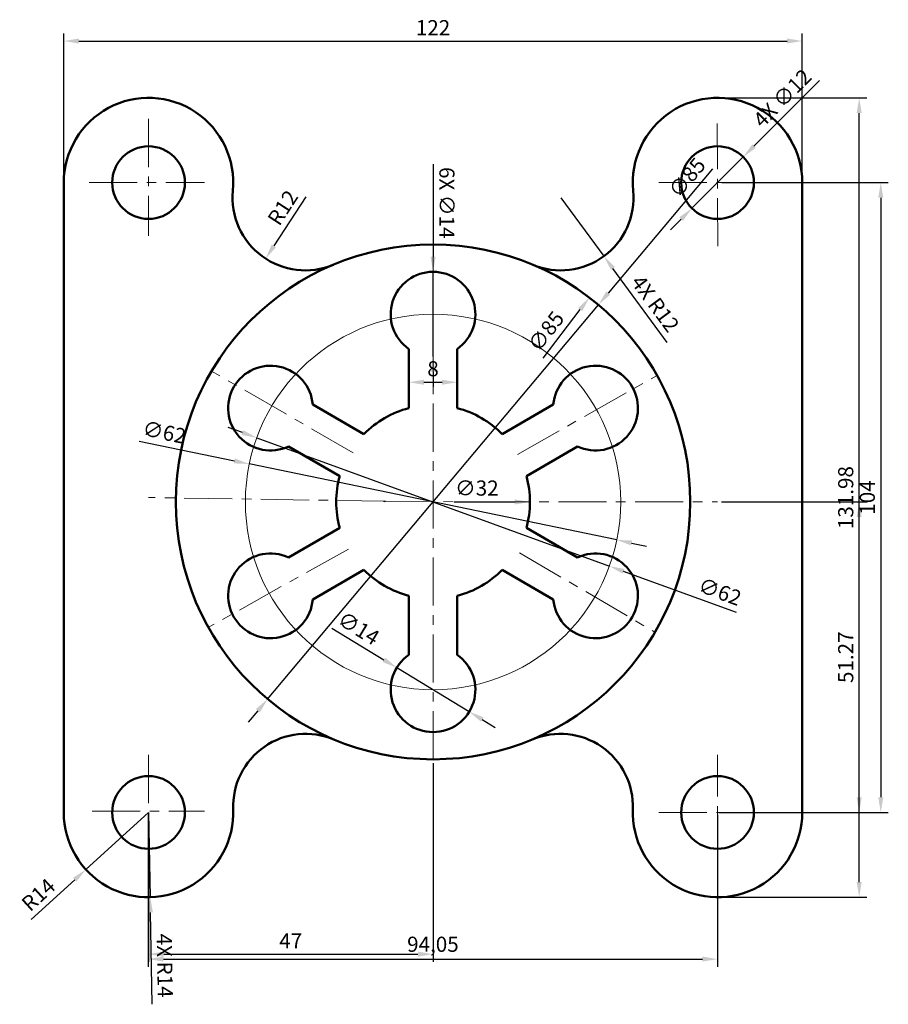
# Model space of a CAD drawing. Units: millimetres. Extents: x 2270 to 2413, y 909 to 1072.
import ezdxf

# ---------------------------------------------------------------- set-up
doc = ezdxf.new("R2010")
doc.units = ezdxf.units.MM
doc.linetypes.add('CENTER', pattern=[50.8, 31.75, -6.35, 6.35, -6.35])
for name, color, linetype, lineweight in [('M-CNTR', 4, 'CENTER', 18), ('M-CONS', 8, 'Continuous', 13), ('M-DIMS', 2, 'Continuous', 25), ('M-OUTL', 7, 'Continuous', 50)]:
    doc.layers.add(name, color=color, linetype=linetype, lineweight=lineweight)
doc.styles.get("Standard").update_dxf_attribs({"font": 'arial.ttf'})
doc.dimstyles.new('ISO-25', dxfattribs={"dimtxt": 2.5, "dimasz": 2.5, "dimexe": 1.25, "dimexo": 0.625, "dimtad": 1, "dimtxsty": 'Standard', "dimcen": 2.5, "dimadec": 0, "dimazin": 0, "dimtfac": 1, "dimtmove": 0, "dimatfit": 3, "dimfxl": 1, "dimarcsym": 0})

# ---------------------------------------------------------------- blocks, each defined once
blk = doc.blocks.new('*D1')
at = {"layer": 'Defpoints', "color": 0, "transparency": 16777216}
for p in [(2385.31, 1044.65), (2384.82, 940.65), (2412.2, 940.65)]:
    blk.add_point(p, dxfattribs=at)
at = {"layer": 'M-DIMS', "color": 0, "lineweight": -2, "transparency": 16777216}
for p, q in [((2385.94, 1044.65), (2413.45, 1044.65)), ((2412.2, 1042.15), (2412.2, 943.15)), ((2385.45, 940.65), (2413.45, 940.65))]:
    blk.add_line(p, q, dxfattribs=at)
at = {"layer": 'M-DIMS', "color": 0, "transparency": 16777216}
for points in [[(2411.79, 1042.15), (2412.62, 1042.15), (2412.2, 1044.65)], [(2411.79, 943.15), (2412.62, 943.15), (2412.2, 940.65)]]:
    blk.add_solid(points, dxfattribs=at)
at = {"layer": 'M-DIMS', "color": 0, "transparency": 16777216, "insert": (2410.3, 992.65), "char_height": 2.5, "attachment_point": 5, "rotation": 90}
blk.add_mtext('104', dxfattribs=at)
blk = doc.blocks.new('*D2')
at = {"layer": 'Defpoints', "color": 0, "transparency": 16777216}
for p in [(2291.19, 940.86), (2385.24, 940.86), (2385.24, 916.43)]:
    blk.add_point(p, dxfattribs=at)
at = {"layer": 'M-DIMS', "color": 0, "lineweight": -2, "transparency": 16777216}
for p, q in [((2291.19, 940.23), (2291.19, 915.18)), ((2385.24, 940.23), (2385.24, 915.18)), ((2293.69, 916.43), (2382.74, 916.43))]:
    blk.add_line(p, q, dxfattribs=at)
at = {"layer": 'M-DIMS', "color": 0, "transparency": 16777216}
for points in [[(2293.69, 916.85), (2293.69, 916.02), (2291.19, 916.43)], [(2382.74, 916.85), (2382.74, 916.02), (2385.24, 916.43)]]:
    blk.add_solid(points, dxfattribs=at)
at = {"layer": 'M-DIMS', "color": 0, "transparency": 16777216, "insert": (2338.22, 918.56), "char_height": 2.5, "attachment_point": 5}
blk.add_mtext('94,05', dxfattribs=at)
blk = doc.blocks.new('*D3')
at = {"layer": 'Defpoints', "color": 0, "transparency": 16777216}
for p in [(2334.24, 1012.29), (2342.24, 1012.29), (2342.24, 1011.69)]:
    blk.add_point(p, dxfattribs=at)
at = {"layer": 'M-DIMS', "color": 0, "lineweight": -2, "transparency": 16777216}
for p, q in [((2334.24, 1011.67), (2334.24, 1010.44)), ((2336.74, 1011.69), (2339.74, 1011.69)), ((2342.24, 1011.67), (2342.24, 1010.44))]:
    blk.add_line(p, q, dxfattribs=at)
at = {"layer": 'M-DIMS', "color": 0, "transparency": 16777216}
for points in [[(2336.74, 1012.1), (2336.74, 1011.27), (2334.24, 1011.69)], [(2339.74, 1012.1), (2339.74, 1011.27), (2342.24, 1011.69)]]:
    blk.add_solid(points, dxfattribs=at)
at = {"layer": 'M-DIMS', "color": 0, "transparency": 16777216, "insert": (2338.24, 1013.59), "char_height": 2.5, "attachment_point": 5}
blk.add_mtext('8', dxfattribs=at)
blk = doc.blocks.new('*D4')
at = {"layer": 'Defpoints', "color": 0, "transparency": 16777216}
for p in [(2317.12, 1042.16), (2310.58, 1032.1)]:
    blk.add_point(p, dxfattribs=at)
at = {"layer": 'M-DIMS', "color": 0, "lineweight": -2, "transparency": 16777216}
blk.add_line((2317.23, 1042.33), (2311.94, 1034.2), dxfattribs=at)
at = {"layer": 'M-DIMS', "color": 0, "transparency": 16777216}
blk.add_solid([(2311.59, 1034.43), (2312.29, 1033.97), (2310.58, 1032.1)], dxfattribs=at)
at = {"layer": 'M-DIMS', "color": 0, "transparency": 16777216, "insert": (2313.69, 1040.34), "char_height": 2.5, "attachment_point": 5, "rotation": 56.9544}
blk.add_mtext('R12', dxfattribs=at)
blk = doc.blocks.new('*D5')
at = {"layer": 'Defpoints', "color": 0, "transparency": 16777216}
for p in [(2291.24, 940.65), (2280.89, 931.22)]:
    blk.add_point(p, dxfattribs=at)
at = {"layer": 'M-DIMS', "color": 0, "lineweight": -2, "transparency": 16777216}
for p, q in [((2291.24, 940.65), (2280.89, 931.22)), ((2271.86, 923), (2279.04, 929.54))]:
    blk.add_line(p, q, dxfattribs=at)
at = {"layer": 'M-DIMS', "color": 0, "transparency": 16777216}
blk.add_solid([(2278.76, 929.85), (2279.32, 929.23), (2280.89, 931.22)], dxfattribs=at)
at = {"layer": 'M-DIMS', "color": 0, "transparency": 16777216, "insert": (2273.26, 926.82), "char_height": 2.5, "attachment_point": 5, "rotation": 42.3158}
blk.add_mtext('R14', dxfattribs=at)
blk = doc.blocks.new('*D6')
at = {"layer": 'Defpoints', "color": 0, "transparency": 16777216}
for p in [(2364.07, 1025.67), (2312.41, 958.17)]:
    blk.add_point(p, dxfattribs=at)
at = {"layer": 'M-DIMS', "color": 0, "lineweight": -2, "transparency": 16777216}
blk.add_line((2356.43, 1015.69), (2362.56, 1023.68), dxfattribs=at)
at = {"layer": 'M-DIMS', "color": 0, "transparency": 16777216}
blk.add_solid([(2362.22, 1023.94), (2362.89, 1023.43), (2364.07, 1025.67)], dxfattribs=at)
at = {"layer": 'M-DIMS', "color": 0, "transparency": 16777216, "insert": (2357.17, 1019.89), "char_height": 2.5, "attachment_point": 5, "rotation": 52.5647}
blk.add_mtext('∅85', dxfattribs=at)
blk = doc.blocks.new('*D7')
at = {"layer": 'Defpoints', "color": 0, "transparency": 16777216}
for p in [(2322.24, 991.92), (2354.24, 991.92)]:
    blk.add_point(p, dxfattribs=at)
at = {"layer": 'M-DIMS', "color": 0, "lineweight": -2, "transparency": 16777216}
blk.add_line((2341.71, 991.92), (2351.74, 991.92), dxfattribs=at)
at = {"layer": 'M-DIMS', "color": 0, "transparency": 16777216}
blk.add_solid([(2351.74, 992.34), (2351.74, 991.5), (2354.24, 991.92)], dxfattribs=at)
at = {"layer": 'M-DIMS', "color": 0, "transparency": 16777216, "insert": (2345.48, 993.89), "char_height": 2.5, "attachment_point": 5}
blk.add_mtext('∅32', dxfattribs=at)
blk = doc.blocks.new('*D8')
at = {"layer": 'Defpoints', "color": 0, "transparency": 16777216}
for p in [(2332.26, 964.55), (2344.22, 957.29)]:
    blk.add_point(p, dxfattribs=at)
at = {"layer": 'M-DIMS', "color": 0, "lineweight": -2, "transparency": 16777216}
for p, q in [((2321.54, 971.06), (2330.12, 965.85)), ((2344.22, 957.29), (2332.26, 964.55)), ((2346.36, 955.99), (2348.5, 954.69))]:
    blk.add_line(p, q, dxfattribs=at)
at = {"layer": 'M-DIMS', "color": 0, "transparency": 16777216}
for points in [[(2330.34, 966.21), (2329.9, 965.49), (2332.26, 964.55)], [(2346.58, 956.35), (2346.15, 955.64), (2344.22, 957.29)]]:
    blk.add_solid(points, dxfattribs=at)
at = {"layer": 'M-DIMS', "color": 0, "transparency": 16777216, "insert": (2325.78, 970.79), "char_height": 2.5, "attachment_point": 5, "rotation": 328.7451}
blk.add_mtext('∅14', dxfattribs=at)
blk = doc.blocks.new('*D9')
at = {"layer": 'Defpoints', "color": 0, "transparency": 16777216}
for p in [(2307.88, 998.19), (2368.6, 985.65)]:
    blk.add_point(p, dxfattribs=at)
at = {"layer": 'M-DIMS', "color": 0, "lineweight": -2, "transparency": 16777216}
for p, q in [((2289.71, 1001.94), (2305.43, 998.7)), ((2368.6, 985.65), (2307.88, 998.19)), ((2371.05, 985.14), (2373.5, 984.64))]:
    blk.add_line(p, q, dxfattribs=at)
at = {"layer": 'M-DIMS', "color": 0, "transparency": 16777216}
for points in [[(2305.52, 999.1), (2305.35, 998.29), (2307.88, 998.19)], [(2371.13, 985.55), (2370.96, 984.74), (2368.6, 985.65)]]:
    blk.add_solid(points, dxfattribs=at)
at = {"layer": 'M-DIMS', "color": 0, "transparency": 16777216, "insert": (2293.79, 1003.11), "char_height": 2.5, "attachment_point": 5, "rotation": 348.3297}
blk.add_mtext('∅62', dxfattribs=at)
blk = doc.blocks.new('MOUNTING-HOLE-D12')
blk.add_circle((6, 6), 6)
blk = doc.blocks.new('*D11')
at = {"layer": 'Defpoints', "color": 0, "transparency": 16777216}
for p in [(2399.24, 1068.03), (2277.24, 1044.65), (2399.24, 1044.65)]:
    blk.add_point(p, dxfattribs=at)
at = {"layer": 'M-DIMS', "color": 0, "lineweight": -2, "transparency": 16777216}
for p, q in [((2277.24, 1045.27), (2277.24, 1069.28)), ((2399.24, 1045.27), (2399.24, 1069.28)), ((2279.74, 1068.03), (2396.74, 1068.03))]:
    blk.add_line(p, q, dxfattribs=at)
at = {"layer": 'M-DIMS', "color": 0, "transparency": 16777216}
for points in [[(2279.74, 1068.45), (2279.74, 1067.62), (2277.24, 1068.03)], [(2396.74, 1068.45), (2396.74, 1067.62), (2399.24, 1068.03)]]:
    blk.add_solid(points, dxfattribs=at)
at = {"layer": 'M-DIMS', "color": 0, "transparency": 16777216, "insert": (2338.24, 1069.91), "char_height": 2.5, "attachment_point": 5}
blk.add_mtext('122', dxfattribs=at)
blk = doc.blocks.new('*D12')
at = {"layer": 'Defpoints', "color": 0, "transparency": 16777216}
for p in [(2385.24, 991.92), (2408.64, 991.92), (2399.24, 940.65)]:
    blk.add_point(p, dxfattribs=at)
at = {"layer": 'M-DIMS', "color": 0, "lineweight": -2, "transparency": 16777216}
for p, q in [((2385.87, 991.92), (2409.89, 991.92)), ((2408.64, 943.15), (2408.64, 989.42)), ((2399.87, 940.65), (2409.89, 940.65))]:
    blk.add_line(p, q, dxfattribs=at)
at = {"layer": 'M-DIMS', "color": 0, "transparency": 16777216}
for points in [[(2408.22, 989.42), (2409.06, 989.42), (2408.64, 991.92)], [(2408.22, 943.15), (2409.06, 943.15), (2408.64, 940.65)]]:
    blk.add_solid(points, dxfattribs=at)
at = {"layer": 'M-DIMS', "color": 0, "transparency": 16777216, "insert": (2406.74, 966.28), "char_height": 2.5, "attachment_point": 5, "rotation": 90}
blk.add_mtext('51.27', dxfattribs=at)
blk = doc.blocks.new('*D13')
at = {"layer": 'Defpoints', "color": 0, "transparency": 16777216}
for p in [(2384.57, 1058.63), (2408.64, 1058.63), (2384.97, 926.65)]:
    blk.add_point(p, dxfattribs=at)
at = {"layer": 'M-DIMS', "color": 0, "lineweight": -2, "transparency": 16777216}
for p, q in [((2385.2, 1058.63), (2409.89, 1058.63)), ((2408.64, 929.15), (2408.64, 1056.13)), ((2385.6, 926.65), (2409.89, 926.65))]:
    blk.add_line(p, q, dxfattribs=at)
at = {"layer": 'M-DIMS', "color": 0, "transparency": 16777216}
for points in [[(2408.22, 1056.13), (2409.06, 1056.13), (2408.64, 1058.63)], [(2408.22, 929.15), (2409.06, 929.15), (2408.64, 926.65)]]:
    blk.add_solid(points, dxfattribs=at)
at = {"layer": 'M-DIMS', "color": 0, "transparency": 16777216, "insert": (2406.74, 992.64), "char_height": 2.5, "attachment_point": 5, "rotation": 90}
blk.add_mtext('131.98', dxfattribs=at)
blk = doc.blocks.new('*D14')
at = {"layer": 'Defpoints', "color": 0, "transparency": 16777216}
for p in [(2338.24, 949.42), (2291.24, 934.65), (2338.24, 917.25)]:
    blk.add_point(p, dxfattribs=at)
at = {"layer": 'M-DIMS', "color": 0, "lineweight": -2, "transparency": 16777216}
for p, q in [((2338.24, 948.8), (2338.24, 916)), ((2291.24, 934.02), (2291.24, 916)), ((2293.74, 917.25), (2335.74, 917.25))]:
    blk.add_line(p, q, dxfattribs=at)
at = {"layer": 'M-DIMS', "color": 0, "transparency": 16777216}
for points in [[(2293.74, 917.67), (2293.74, 916.83), (2291.24, 917.25)], [(2335.74, 917.67), (2335.74, 916.83), (2338.24, 917.25)]]:
    blk.add_solid(points, dxfattribs=at)
at = {"layer": 'M-DIMS', "color": 0, "transparency": 16777216, "insert": (2314.74, 919.13), "char_height": 2.5, "attachment_point": 5}
blk.add_mtext('47', dxfattribs=at)
blk = doc.blocks.new('*D15')
at = {"layer": 'Defpoints', "color": 0, "transparency": 16777216}
for p in [(2309.11, 1002.52), (2367.37, 981.32)]:
    blk.add_point(p, dxfattribs=at)
at = {"layer": 'M-DIMS', "color": 0, "lineweight": -2, "transparency": 16777216}
for p, q in [((2306.76, 1003.38), (2304.41, 1004.23)), ((2309.11, 1002.52), (2367.37, 981.32)), ((2388.38, 973.67), (2369.72, 980.46))]:
    blk.add_line(p, q, dxfattribs=at)
at = {"layer": 'M-DIMS', "color": 0, "transparency": 16777216}
for points in [[(2306.9, 1003.77), (2306.62, 1002.99), (2309.11, 1002.52)], [(2369.86, 980.85), (2369.58, 980.07), (2367.37, 981.32)]]:
    blk.add_solid(points, dxfattribs=at)
at = {"layer": 'M-DIMS', "color": 0, "transparency": 16777216, "insert": (2385.52, 976.81), "char_height": 2.5, "attachment_point": 5, "rotation": 339.9972}
blk.add_mtext('∅62', dxfattribs=at)
blk = doc.blocks.new('*D16')
at = {"layer": 'Defpoints', "color": 0, "transparency": 16777216}
for p in [(2365.56, 1024.47), (2310.92, 959.37)]:
    blk.add_point(p, dxfattribs=at)
at = {"layer": 'M-DIMS', "color": 0, "lineweight": -2, "transparency": 16777216}
for p, q in [((2384.39, 1046.9), (2367.17, 1026.39)), ((2310.92, 959.37), (2365.56, 1024.47)), ((2309.31, 957.45), (2307.7, 955.54))]:
    blk.add_line(p, q, dxfattribs=at)
at = {"layer": 'M-DIMS', "color": 0, "transparency": 16777216}
for points in [[(2366.85, 1026.66), (2367.49, 1026.12), (2365.56, 1024.47)], [(2308.99, 957.72), (2309.63, 957.18), (2310.92, 959.37)]]:
    blk.add_solid(points, dxfattribs=at)
at = {"layer": 'M-DIMS', "color": 0, "transparency": 16777216, "insert": (2380.45, 1045.27), "char_height": 2.5, "attachment_point": 5, "rotation": 49.9927}
blk.add_mtext('∅85', dxfattribs=at)
blk = doc.blocks.new('*D17')
at = {"layer": 'Defpoints', "color": 0, "transparency": 16777216}
for p in [(2338.24, 1029.92), (2338.24, 1015.92)]:
    blk.add_point(p, dxfattribs=at)
at = {"layer": 'M-DIMS', "color": 0, "lineweight": -2, "transparency": 16777216}
for p, q in [((2338.24, 1047.71), (2338.24, 1032.42)), ((2338.24, 1015.92), (2338.24, 1029.92)), ((2338.24, 1013.42), (2338.24, 1010.92))]:
    blk.add_line(p, q, dxfattribs=at)
at = {"layer": 'M-DIMS', "color": 0, "transparency": 16777216}
for points in [[(2338.66, 1032.42), (2337.82, 1032.42), (2338.24, 1029.92)], [(2338.66, 1013.42), (2337.82, 1013.42), (2338.24, 1015.92)]]:
    blk.add_solid(points, dxfattribs=at)
at = {"layer": 'M-DIMS', "color": 0, "transparency": 16777216, "insert": (2340.21, 1041.32), "char_height": 2.5, "attachment_point": 5, "rotation": 270.0036}
blk.add_mtext('6X ∅14', dxfattribs=at)
blk = doc.blocks.new('*D18')
at = {"layer": 'Defpoints', "color": 0, "transparency": 16777216}
for p in [(2291.24, 940.65), (2291.51, 926.65)]:
    blk.add_point(p, dxfattribs=at)
at = {"layer": 'M-DIMS', "color": 0, "lineweight": -2, "transparency": 16777216}
for p, q in [((2291.24, 940.65), (2291.51, 926.65)), ((2291.84, 908.97), (2291.55, 924.15))]:
    blk.add_line(p, q, dxfattribs=at)
at = {"layer": 'M-DIMS', "color": 0, "transparency": 16777216}
blk.add_solid([(2291.97, 924.16), (2291.14, 924.14), (2291.51, 926.65)], dxfattribs=at)
at = {"layer": 'M-DIMS', "color": 0, "transparency": 16777216, "insert": (2293.6, 915.35), "char_height": 2.5, "attachment_point": 5, "rotation": 271.0868}
blk.add_mtext('4X R14', dxfattribs=at)
blk = doc.blocks.new('*D19')
at = {"layer": 'Defpoints', "color": 0, "transparency": 16777216}
for p in [(2359.36, 1042.16), (2366.47, 1032.5)]:
    blk.add_point(p, dxfattribs=at)
at = {"layer": 'M-DIMS', "color": 0, "lineweight": -2, "transparency": 16777216}
for p, q in [((2359.36, 1042.16), (2366.47, 1032.5)), ((2376.94, 1018.26), (2367.95, 1030.48))]:
    blk.add_line(p, q, dxfattribs=at)
at = {"layer": 'M-DIMS', "color": 0, "transparency": 16777216}
blk.add_solid([(2368.29, 1030.73), (2367.62, 1030.24), (2366.47, 1032.5)], dxfattribs=at)
at = {"layer": 'M-DIMS', "color": 0, "transparency": 16777216, "insert": (2374.7, 1024.48), "char_height": 2.5, "attachment_point": 5, "rotation": 306.3423}
blk.add_mtext('4X R12', dxfattribs=at)
blk = doc.blocks.new('*D20')
at = {"layer": 'Defpoints', "color": 0, "transparency": 16777216}
for p in [(2389.48, 1048.89), (2381, 1040.41)]:
    blk.add_point(p, dxfattribs=at)
at = {"layer": 'M-DIMS', "color": 0, "lineweight": -2, "transparency": 16777216}
for p, q in [((2402.11, 1061.53), (2391.25, 1050.66)), ((2381, 1040.41), (2389.48, 1048.89)), ((2379.23, 1038.64), (2377.46, 1036.87))]:
    blk.add_line(p, q, dxfattribs=at)
at = {"layer": 'M-DIMS', "color": 0, "transparency": 16777216}
for points in [[(2390.96, 1050.95), (2391.54, 1050.37), (2389.48, 1048.89)], [(2378.94, 1038.93), (2379.53, 1038.34), (2381, 1040.41)]]:
    blk.add_solid(points, dxfattribs=at)
at = {"layer": 'M-DIMS', "color": 0, "transparency": 16777216, "insert": (2396.17, 1058.37), "char_height": 2.5, "attachment_point": 5, "rotation": 45.0106}
blk.add_mtext('4X ∅12', dxfattribs=at)

msp = doc.modelspace()

# ---------------------------------------------------------------- linework, layer by layer
at = {"layer": 'M-CNTR', "ltscale": 0.25}
for p, q in [((2291.24, 1055.159), (2291.24, 1035.865)), ((2385.311, 1034.155), (2385.175, 1054.435)), ((2281.414, 1044.649), (2300.482, 1044.649)), ((2375.532, 1044.649), (2395.089, 1044.649)), ((2338.24, 949.42), (2338.24, 1034.42)), ((2325.04, 1000.039), (2301.652, 1013.542)), ((2352.176, 999.781), (2375.257, 1012.801)), ((2330.45, 992.041), (2291.24, 992.649)), ((2330.45, 992.041), (2346.24, 991.92)), ((2346.24, 991.92), (2385.24, 991.92)), ((2324.267, 984.127), (2301.123, 971.219)), ((2352.519, 983.54), (2374.894, 970.408)), ((2291.24, 950.139), (2291.24, 931.577)), ((2385.24, 930.6), (2385.24, 950.139)), ((2281.903, 940.858), (2300.482, 940.858)), ((2375.532, 940.649), (2394.112, 940.649))]:
    msp.add_line(p, q, dxfattribs=at)
at = {"layer": 'M-CONS'}
for p, q in [((2330.24, 991.92), (2330.02, 992.048)), ((2330.45, 992.041), (2330.24, 991.92))]:
    msp.add_line(p, q, dxfattribs=at)
msp.add_circle((2338.24, 991.92), 31, dxfattribs=at)
at = {"layer": 'M-OUTL'}
for p, q in [((2277.24, 940.649), (2277.24, 1044.649)), ((2399.24, 940.649), (2399.24, 1044.649)), ((2334.24, 1007.412), (2334.24, 1017.176)), ((2342.24, 1007.412), (2342.24, 1017.176)), ((2326.824, 1003.13), (2318.369, 1008.012)), ((2349.657, 1003.13), (2358.112, 1008.012)), ((2322.824, 996.202), (2314.369, 1001.084)), ((2353.657, 996.202), (2362.112, 1001.084)), ((2322.824, 987.638), (2314.369, 982.757)), ((2353.657, 987.638), (2362.112, 982.757)), ((2326.824, 980.71), (2318.369, 975.828)), ((2349.657, 980.71), (2358.112, 975.828)), ((2334.24, 966.665), (2334.24, 976.428)), ((2342.24, 966.665), (2342.24, 976.428))]:
    msp.add_line(p, q, dxfattribs=at)
msp.add_circle((2338.24, 991.92), 42.5, dxfattribs=at)
for centre, radius, start, end in [((2291.24, 1044.649), 14, 354.51126, 180), ((2385.24, 1044.649), 14, 0, 185.48874), ((2317.121, 1042.162), 12, 174.51126, 292.79956), ((2359.36, 1042.162), 12, 247.20044, 5.48874), ((2338.24, 1022.92), 7, 304.8499, 235.1501), ((2311.394, 1007.42), 7, 4.8499, 295.1501), ((2365.087, 1007.42), 7, 244.8499, 175.1501), ((2338.24, 991.92), 16, 104.47751, 135.52249), ((2338.24, 991.92), 16, 44.47751, 75.52249), ((2338.24, 991.92), 16, 164.47751, 195.52249), ((2338.24, 991.92), 16, 344.47751, 15.52249), ((2311.394, 976.42), 7, 64.8499, 355.1501), ((2365.087, 976.42), 7, 184.8499, 115.1501), ((2338.24, 991.92), 16, 224.47751, 255.52249), ((2338.24, 991.92), 16, 284.47751, 315.52249), ((2338.24, 960.92), 7, 124.8499, 55.1501), ((2317.222, 941.636), 12, 67.31495, 182.17684), ((2359.259, 941.636), 12, 357.82316, 112.68505), ((2291.24, 940.649), 14, 180, 2.17684), ((2385.24, 940.649), 14, 177.82316, 0)]:
    msp.add_arc(centre, radius, start, end, dxfattribs=at)

# ---------------------------------------------------------------- block references
for p in [(2285.24, 1038.649), (2379.24, 1038.649), (2285.24, 934.649), (2379.24, 934.649)]:
    msp.add_blockref('MOUNTING-HOLE-D12', p, dxfattribs=at)

# ---------------------------------------------------------------- dimensions: what is measured, and where the dimension line sits
at = {"layer": 'M-DIMS'}
for base, p1, p2, override, picture, middle in [((2399.24, 1068.033), (2277.24, 1044.649), (2399.24, 1044.649), {"dimdec": 0, "dimlfac": 1, "dimrnd": 0, "dimzin": 0, "dimdsep": 46, "dimlunit": 2}, '*D11', (2338.24, 1069.913)), ((2342.24, 1011.686), (2334.24, 1012.294), (2342.24, 1012.294), {"dimclrd": 0, "dimclre": 0, "dimclrt": 0}, '*D3', (2338.24, 1013.587)), ((2338.24, 917.251), (2291.24, 934.649), (2338.24, 949.42), {"dimdec": 0, "dimlfac": 1, "dimrnd": 0, "dimzin": 0, "dimdsep": 46, "dimlunit": 2}, '*D14', (2314.74, 919.126)), ((2385.24, 916.434), (2291.193, 940.858), (2385.24, 940.858), {"dimclrd": 0, "dimclre": 0, "dimclrt": 0}, '*D2', (2338.217, 918.562))]:
    dim = msp.add_linear_dim(base=base, p1=p1, p2=p2, dimstyle='ISO-25', override=override, dxfattribs=at)
    dim.commit()
    dim.dimension.update_dxf_attribs({"geometry": picture, "text_midpoint": middle})
for p1, p2, text, picture, middle in [((2380.999, 1040.405), (2389.482, 1048.892), '4X <>', '*D20', (2397.565, 1056.978)), ((2338.241, 1015.92), (2338.24, 1029.92), '6X <>', '*D17', (2338.239, 1041.317))]:
    dim = msp.add_diameter_dim_2p(p1=p1, p2=p2, text=text, dimstyle='ISO-25', override={"dimdec": 0, "dimlfac": 1, "dimrnd": 0, "dimzin": 0, "dimdsep": 46, "dimlunit": 2}, dxfattribs=at)
    dim.commit()
    dim.dimension.update_dxf_attribs({"geometry": picture, "text_midpoint": middle, "dimtype": 163})
for base, p1, p2, override, picture, middle in [((2408.64, 1058.633), (2384.975, 926.651), (2384.57, 1058.633), {"dimdec": 2, "dimlfac": 1, "dimrnd": 0, "dimzin": 0, "dimdsep": 46, "dimlunit": 2}, '*D13', (2406.738, 992.642)), ((2412.202, 940.649), (2385.311, 1044.649), (2384.822, 940.649), {"dimclrd": 0, "dimclre": 0, "dimclrt": 0}, '*D1', (2410.3, 992.649)), ((2408.64, 991.92), (2399.24, 940.649), (2385.24, 991.92), {"dimdec": 2, "dimlfac": 1, "dimrnd": 0, "dimzin": 0, "dimdsep": 46, "dimlunit": 2}, '*D12', (2406.739, 966.285))]:
    dim = msp.add_linear_dim(base=base, p1=p1, p2=p2, angle=90, dimstyle='ISO-25', override=override, dxfattribs=at)
    dim.commit()
    dim.dimension.update_dxf_attribs({"geometry": picture, "text_midpoint": middle})
for p1, p2, override, picture, middle in [((2310.918, 959.367), (2365.563, 1024.474), {"dimdec": 0, "dimlfac": 1, "dimrnd": 0, "dimzin": 0, "dimdsep": 46, "dimlunit": 2}, '*D16', (2381.957, 1044.006)), ((2312.406, 958.174), (2364.075, 1025.667), {"dimclrd": 0, "dimclre": 0, "dimclrt": 0}, '*D6', (2358.735, 1018.691)), ((2368.6, 985.65), (2307.881, 998.191), {"dimclrd": 0, "dimclre": 0, "dimclrt": 0}, '*D9', (2293.393, 1001.183)), ((2309.11, 1002.524), (2367.37, 981.316), {"dimdec": 0, "dimlfac": 1, "dimrnd": 0, "dimzin": 0, "dimdsep": 46, "dimlunit": 2}, '*D15', (2384.848, 974.954)), ((2322.24, 991.92), (2354.24, 991.92), {"dimclrd": 0, "dimclre": 0, "dimclrt": 0}, '*D7', (2345.478, 991.92))]:
    dim = msp.add_diameter_dim_2p(p1=p1, p2=p2, dimstyle='ISO-25', override=override, dxfattribs=at)
    dim.commit()
    dim.dimension.update_dxf_attribs({"geometry": picture, "text_midpoint": middle, "dimtype": 163})
dim = msp.add_radius_dim(center=(2317.121, 1042.162), mpoint=(2310.578, 1032.103), dimstyle='ISO-25', override={"dimclrd": 0, "dimclre": 0, "dimclrt": 0}, dxfattribs=at)
dim.commit()
dim.dimension.update_dxf_attribs({"geometry": '*D4', "text_midpoint": (2315.267, 1039.311), "dimtype": 164})
for center, mpoint, picture, middle in [((2359.36, 1042.162), (2366.471, 1032.496), '*D19', (2374.703, 1024.48)), ((2291.24, 940.649), (2291.506, 926.651), '*D18', (2293.602, 915.346))]:
    dim = msp.add_radius_dim(center=center, mpoint=mpoint, text='4X <>', dimstyle='ISO-25', override={"dimdec": 0, "dimlfac": 1, "dimrnd": 0, "dimzin": 0, "dimdsep": 46, "dimlunit": 2}, dxfattribs=at)
    dim.commit()
    dim.dimension.update_dxf_attribs({"geometry": picture, "text_midpoint": middle})
dim = msp.add_diameter_dim_2p(p1=(2344.225, 957.288), p2=(2332.256, 964.552), dimstyle='ISO-25', override={"dimclrd": 0, "dimclre": 0, "dimclrt": 0}, dxfattribs=at)
dim.commit()
dim.dimension.update_dxf_attribs({"geometry": '*D8', "text_midpoint": (2325.782, 970.788)})
dim = msp.add_radius_dim(center=(2291.24, 940.649), mpoint=(2280.888, 931.224), dimstyle='ISO-25', override={"dimclrd": 0, "dimclre": 0, "dimclrt": 0}, dxfattribs=at)
dim.commit()
dim.dimension.update_dxf_attribs({"geometry": '*D5', "text_midpoint": (2273.258, 926.82)})

doc.saveas('drawing.dxf')
